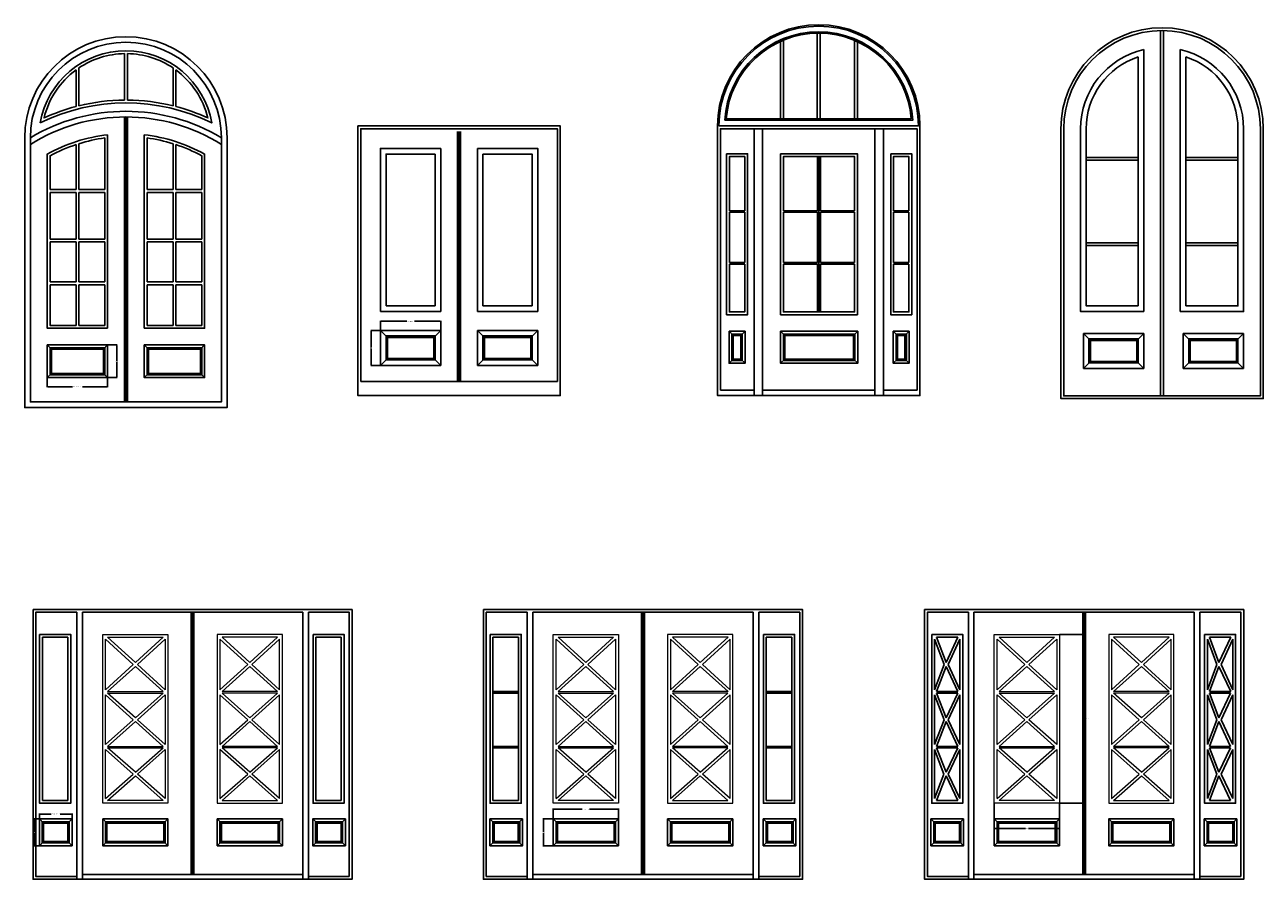
# Model space of a CAD drawing. Units: inches. Extents: x 1451 to 1892, y 1255 to 1559.
import ezdxf

# ---------------------------------------------------------------- set-up
doc = ezdxf.new("R2010")
doc.units = ezdxf.units.IN
doc.header["$MEASUREMENT"] = 0
for name, color, linetype, lineweight in [('A-ANNO-DIMS', 2, 'Continuous', 18), ('A-DOOR', 4, 'Continuous', 25), ('A-GLAZ', 3, 'Continuous', 18)]:
    doc.layers.add(name, color=color, linetype=linetype, lineweight=lineweight)
doc.styles.get("Standard").update_dxf_attribs({"font": 'arial.ttf'})
doc.dimstyles.get("Standard").update_dxf_attribs({"dimtxt": 0.18, "dimasz": 0.18, "dimexe": 0.18, "dimexo": 0.0625, "dimgap": 0.09, "dimtad": 0, "dimtih": 1, "dimtoh": 1, "dimdec": 4, "dimzin": 0, "dimdsep": 46, "dimtxsty": 'Standard', "dimcen": 0.09, "dimadec": 0, "dimazin": 0, "dimtfac": 1, "dimtdec": 4, "dimtofl": 0, "dimtmove": 0, "dimatfit": 3, "dimfxl": 1, "dimtolj": 1, "dimtzin": 0, "dimarcsym": 0})

# ---------------------------------------------------------------- blocks, each defined once
blk = doc.blocks.new('GLAZ-X-MUNTIN')
for p, q in [((1489.65, 1331.77), (1479.78, 1340.77)), ((1490.39, 1332.44), (1480.52, 1341.44)), ((1490.39, 1332.44), (1500.26, 1341.44)), ((1491.13, 1331.77), (1501, 1340.77)), ((1479.78, 1322.77), (1489.65, 1331.77)), ((1480.52, 1322.09), (1490.39, 1331.09)), ((1500.26, 1322.09), (1490.39, 1331.09)), ((1501, 1322.77), (1491.13, 1331.77)), ((1480.52, 1322.09), (1500.26, 1322.09)), ((1489.64, 1312.11), (1479.78, 1320.92)), ((1480.53, 1321.59), (1500.25, 1321.59)), ((1490.39, 1312.78), (1480.53, 1321.59)), ((1490.39, 1312.78), (1500.25, 1321.59)), ((1491.14, 1312.11), (1501, 1320.92)), ((1479.78, 1303.29), (1489.64, 1312.11)), ((1480.53, 1302.62), (1490.39, 1311.44)), ((1500.25, 1302.62), (1490.39, 1311.44)), ((1501, 1303.29), (1491.14, 1312.11)), ((1489.64, 1292.74), (1479.78, 1301.46)), ((1480.53, 1302.62), (1500.25, 1302.62)), ((1480.54, 1302.12), (1500.24, 1302.12)), ((1490.39, 1293.41), (1480.54, 1302.12)), ((1490.39, 1293.41), (1500.24, 1302.12)), ((1491.14, 1292.74), (1501, 1301.46)), ((1479.78, 1284.02), (1489.64, 1292.74)), ((1480.54, 1283.35), (1490.39, 1292.07)), ((1500.24, 1283.35), (1490.39, 1292.07)), ((1501, 1284.02), (1491.14, 1292.74))]:
    blk.add_line(p, q)
blk.add_lwpolyline([(1478.78, 1342.44), (1502, 1342.44), (1502, 1282.35), (1478.78, 1282.35)], close=True)
for points in [[(1479.78, 1322.77), (1479.78, 1340.77)], [(1480.52, 1341.44), (1500.26, 1341.44)], [(1501, 1340.77), (1501, 1322.77)], [(1479.78, 1303.29), (1479.78, 1320.92)], [(1501, 1320.92), (1501, 1303.29)], [(1479.78, 1284.02), (1479.78, 1301.46)], [(1501, 1301.46), (1501, 1284.02)], [(1500.24, 1283.35), (1480.54, 1283.35)]]:
    blk.add_lwpolyline(points)
blk = doc.blocks.new('PANEL-RAISED-LEAF')
for p, q in [((1478.78, 1276.79), (1480.28, 1275.29)), ((1502, 1276.79), (1500.5, 1275.29)), ((1478.78, 1267.24), (1480.28, 1268.74)), ((1500.5, 1268.74), (1502, 1267.24))]:
    blk.add_line(p, q)
for points in [[(1478.78, 1276.79), (1502, 1276.79), (1502, 1267.24), (1478.78, 1267.24)], [(1479.78, 1275.79), (1501, 1275.79), (1501, 1268.24), (1479.78, 1268.24)], [(1480.28, 1275.29), (1500.5, 1275.29), (1500.5, 1268.74), (1480.28, 1268.74)]]:
    blk.add_lwpolyline(points, close=True)
blk = doc.blocks.new('PANEL-RAISED-SIDELT')
for p, q in [((1456.26, 1276.79), (1457.76, 1275.29)), ((1467.87, 1276.79), (1466.37, 1275.29)), ((1456.26, 1267.24), (1457.76, 1268.74)), ((1467.87, 1267.24), (1466.37, 1268.74))]:
    blk.add_line(p, q)
for points in [[(1467.87, 1276.79), (1456.26, 1276.79), (1456.26, 1267.24), (1467.87, 1267.24)], [(1466.87, 1275.79), (1457.26, 1275.79), (1457.26, 1268.24), (1466.87, 1268.24)], [(1466.37, 1275.29), (1457.76, 1275.29), (1457.76, 1268.74), (1466.37, 1268.74)]]:
    blk.add_lwpolyline(points, close=True)
blk = doc.blocks.new('PANEL-RAISED-ARCH')
for p, q in [((1459.04, 1445.5), (1460.54, 1444)), ((1480.54, 1445.5), (1479.04, 1444)), ((1459.04, 1433.86), (1460.54, 1435.36)), ((1480.54, 1433.86), (1479.04, 1435.36))]:
    blk.add_line(p, q)
for points in [[(1459.04, 1445.5), (1480.54, 1445.5), (1480.54, 1433.86), (1459.04, 1433.86)], [(1460.04, 1444.5), (1479.54, 1444.5), (1479.54, 1434.86), (1460.04, 1434.86)], [(1460.54, 1444), (1479.04, 1444), (1479.04, 1435.36), (1460.54, 1435.36)]]:
    blk.add_lwpolyline(points, close=True)
blk = doc.blocks.new('PANEL-RAISED-DEEP')
for p, q in [((0, 12.55), (21.5, 12.55)), ((2.5, 10.05), (0, 12.55)), ((21.5, 12.55), (19, 10.05)), ((21.5, 0), (21.5, 12.55)), ((0, 0), (2.5, 2.5)), ((0, 0), (21.5, 0)), ((21.5, 0), (19, 2.5))]:
    blk.add_line(p, q)
blk.add_lwpolyline([(0, 0), (0, 12.55)])
blk.add_lwpolyline([(19, 10.05), (19, 2.5), (2.5, 2.5), (2.5, 10.05)], close=True)
blk = doc.blocks.new('*D6')
at = {"layer": 'A-ANNO-DIMS', "color": 0, "lineweight": -2, "transparency": 16777216}
for p, q in [((1819.28, 1342.44), (1828.41, 1342.44)), ((1828.23, 1342.26), (1828.23, 1312.58)), ((1828.23, 1282.53), (1828.23, 1312.22)), ((1819.28, 1282.35), (1828.41, 1282.35))]:
    blk.add_line(p, q, dxfattribs=at)
at = {"layer": 'A-ANNO-DIMS', "color": 0, "transparency": 16777216}
for points in [[(1828.2, 1342.26), (1828.26, 1342.26), (1828.23, 1342.44)], [(1828.2, 1282.53), (1828.26, 1282.53), (1828.23, 1282.35)]]:
    blk.add_solid(points, dxfattribs=at)
at = {"layer": 'Defpoints', "color": 0, "transparency": 16777216}
for p in [(1819.22, 1342.44), (1828.23, 1342.44), (1819.22, 1282.35)]:
    blk.add_point(p, dxfattribs=at)
at = {"layer": 'A-ANNO-DIMS', "color": 0, "transparency": 16777216, "insert": (1828.23, 1312.4), "char_height": 0.18, "attachment_point": 5}
blk.add_mtext('\\A1;X-MUNTIN LITE 60 TYP.', dxfattribs=at)
blk = doc.blocks.new('*D7')
at = {"layer": 'A-ANNO-DIMS', "color": 0, "lineweight": -2, "transparency": 16777216}
for p, q in [((1796.01, 1282.29), (1796.01, 1273.16)), ((1819.22, 1282.29), (1819.22, 1273.16)), ((1796.19, 1273.34), (1807.08, 1273.34)), ((1819.04, 1273.34), (1808.14, 1273.34))]:
    blk.add_line(p, q, dxfattribs=at)
at = {"layer": 'A-ANNO-DIMS', "color": 0, "transparency": 16777216}
for points in [[(1796.19, 1273.37), (1796.19, 1273.31), (1796.01, 1273.34)], [(1819.04, 1273.37), (1819.04, 1273.31), (1819.22, 1273.34)]]:
    blk.add_solid(points, dxfattribs=at)
at = {"layer": 'Defpoints', "color": 0, "transparency": 16777216}
for p in [(1796.01, 1282.35), (1819.22, 1282.35), (1819.22, 1273.34)]:
    blk.add_point(p, dxfattribs=at)
at = {"layer": 'A-ANNO-DIMS', "color": 0, "transparency": 16777216, "insert": (1807.61, 1273.34), "char_height": 0.18, "attachment_point": 5}
blk.add_mtext('\\A1;23 TYP.', dxfattribs=at)
blk = doc.blocks.new('*D8')
at = {"layer": 'A-ANNO-DIMS', "color": 0, "lineweight": -2, "transparency": 16777216}
for p, q in [((1639.07, 1276.85), (1639.07, 1280.45)), ((1639.25, 1280.27), (1649.36, 1280.27)), ((1662.11, 1280.27), (1652, 1280.27)), ((1662.29, 1276.85), (1662.29, 1280.45))]:
    blk.add_line(p, q, dxfattribs=at)
at = {"layer": 'A-ANNO-DIMS', "color": 0, "transparency": 16777216}
for points in [[(1639.25, 1280.3), (1639.25, 1280.24), (1639.07, 1280.27)], [(1662.11, 1280.3), (1662.11, 1280.24), (1662.29, 1280.27)]]:
    blk.add_solid(points, dxfattribs=at)
at = {"layer": 'Defpoints', "color": 0, "transparency": 16777216}
for p in [(1662.29, 1280.27), (1639.07, 1276.79), (1662.29, 1276.79)]:
    blk.add_point(p, dxfattribs=at)
at = {"layer": 'A-ANNO-DIMS', "color": 0, "transparency": 16777216, "insert": (1650.68, 1280.27), "char_height": 0.18, "attachment_point": 5}
blk.add_mtext('\\A1;LEAF PANEL 23 TYP.', dxfattribs=at)
blk = doc.blocks.new('*D9')
at = {"layer": 'A-ANNO-DIMS', "color": 0, "lineweight": -2, "transparency": 16777216}
for p, q in [((1639.01, 1276.79), (1635.41, 1276.79)), ((1635.59, 1276.61), (1635.59, 1272.2)), ((1635.59, 1267.42), (1635.59, 1271.83)), ((1639.01, 1267.24), (1635.41, 1267.24))]:
    blk.add_line(p, q, dxfattribs=at)
at = {"layer": 'A-ANNO-DIMS', "color": 0, "transparency": 16777216}
for points in [[(1635.56, 1276.61), (1635.62, 1276.61), (1635.59, 1276.79)], [(1635.56, 1267.42), (1635.62, 1267.42), (1635.59, 1267.24)]]:
    blk.add_solid(points, dxfattribs=at)
at = {"layer": 'Defpoints', "color": 0, "transparency": 16777216}
for p in [(1635.59, 1276.79), (1639.07, 1276.79), (1639.07, 1267.24)]:
    blk.add_point(p, dxfattribs=at)
at = {"layer": 'A-ANNO-DIMS', "color": 0, "transparency": 16777216, "insert": (1635.59, 1272.02), "char_height": 0.18, "attachment_point": 5}
blk.add_mtext('\\A1;10 TYP.', dxfattribs=at)
blk = doc.blocks.new('*D10')
at = {"layer": 'A-ANNO-DIMS', "color": 0, "lineweight": -2, "transparency": 16777216}
for p, q in [((1456.26, 1276.85), (1456.26, 1278.71)), ((1456.44, 1278.53), (1460.49, 1278.53)), ((1467.69, 1278.53), (1463.63, 1278.53)), ((1467.87, 1276.85), (1467.87, 1278.71))]:
    blk.add_line(p, q, dxfattribs=at)
at = {"layer": 'A-ANNO-DIMS', "color": 0, "transparency": 16777216}
for points in [[(1456.44, 1278.56), (1456.44, 1278.5), (1456.26, 1278.53)], [(1467.69, 1278.56), (1467.69, 1278.5), (1467.87, 1278.53)]]:
    blk.add_solid(points, dxfattribs=at)
at = {"layer": 'Defpoints', "color": 0, "transparency": 16777216}
for p in [(1467.87, 1278.53), (1456.26, 1276.79), (1467.87, 1276.79)]:
    blk.add_point(p, dxfattribs=at)
at = {"layer": 'A-ANNO-DIMS', "color": 0, "transparency": 16777216, "insert": (1462.06, 1278.53), "char_height": 0.18, "attachment_point": 5}
blk.add_mtext('\\A1;SIDELITE PANEL 12 TYP.', dxfattribs=at)
blk = doc.blocks.new('*D11')
at = {"layer": 'A-ANNO-DIMS', "color": 0, "lineweight": -2, "transparency": 16777216}
for p, q in [((1456.2, 1276.79), (1454.34, 1276.79)), ((1454.52, 1276.61), (1454.52, 1272.2)), ((1454.52, 1267.42), (1454.52, 1271.83)), ((1456.2, 1267.24), (1454.34, 1267.24))]:
    blk.add_line(p, q, dxfattribs=at)
at = {"layer": 'A-ANNO-DIMS', "color": 0, "transparency": 16777216}
for points in [[(1454.49, 1276.61), (1454.55, 1276.61), (1454.52, 1276.79)], [(1454.49, 1267.42), (1454.55, 1267.42), (1454.52, 1267.24)]]:
    blk.add_solid(points, dxfattribs=at)
at = {"layer": 'Defpoints', "color": 0, "transparency": 16777216}
for p in [(1454.52, 1276.79), (1456.26, 1276.79), (1456.26, 1267.24)]:
    blk.add_point(p, dxfattribs=at)
at = {"layer": 'A-ANNO-DIMS', "color": 0, "transparency": 16777216, "insert": (1454.52, 1272.02), "char_height": 0.18, "attachment_point": 5}
blk.add_mtext('\\A1;10 TYP.', dxfattribs=at)
blk = doc.blocks.new('*D12')
at = {"layer": 'A-ANNO-DIMS', "color": 0, "lineweight": -2, "transparency": 16777216}
for p, q in [((1577.58, 1450.74), (1577.58, 1454.09)), ((1577.76, 1453.91), (1586.98, 1453.91)), ((1598.9, 1453.91), (1589.68, 1453.91)), ((1599.08, 1450.74), (1599.08, 1454.09))]:
    blk.add_line(p, q, dxfattribs=at)
at = {"layer": 'A-ANNO-DIMS', "color": 0, "transparency": 16777216}
for points in [[(1577.76, 1453.94), (1577.76, 1453.88), (1577.58, 1453.91)], [(1598.9, 1453.94), (1598.9, 1453.88), (1599.08, 1453.91)]]:
    blk.add_solid(points, dxfattribs=at)
at = {"layer": 'Defpoints', "color": 0, "transparency": 16777216}
for p in [(1577.58, 1450.68), (1599.08, 1453.91), (1599.08, 1450.68)]:
    blk.add_point(p, dxfattribs=at)
at = {"layer": 'A-ANNO-DIMS', "color": 0, "transparency": 16777216, "insert": (1588.33, 1453.91), "char_height": 0.18, "attachment_point": 5}
blk.add_mtext('\\A1;DEEP PANEL 22 TYP.', dxfattribs=at)
blk = doc.blocks.new('*D13')
at = {"layer": 'A-ANNO-DIMS', "color": 0, "lineweight": -2, "transparency": 16777216}
for p, q in [((1577.52, 1450.68), (1574.18, 1450.68)), ((1574.36, 1450.5), (1574.36, 1444.59)), ((1574.36, 1438.31), (1574.36, 1444.22)), ((1577.52, 1438.13), (1574.18, 1438.13))]:
    blk.add_line(p, q, dxfattribs=at)
at = {"layer": 'A-ANNO-DIMS', "color": 0, "transparency": 16777216}
for points in [[(1574.33, 1450.5), (1574.39, 1450.5), (1574.36, 1450.68)], [(1574.33, 1438.31), (1574.39, 1438.31), (1574.36, 1438.13)]]:
    blk.add_solid(points, dxfattribs=at)
at = {"layer": 'Defpoints', "color": 0, "transparency": 16777216}
for p in [(1574.36, 1450.68), (1577.58, 1450.68), (1577.58, 1438.13)]:
    blk.add_point(p, dxfattribs=at)
at = {"layer": 'A-ANNO-DIMS', "color": 0, "transparency": 16777216, "insert": (1574.36, 1444.4), "char_height": 0.18, "attachment_point": 5}
blk.add_mtext('\\A1;13 TYP.', dxfattribs=at)
blk = doc.blocks.new('*D14')
at = {"layer": 'A-ANNO-DIMS', "color": 0, "lineweight": -2, "transparency": 16777216}
for p, q in [((1459.04, 1433.8), (1459.04, 1430.45)), ((1480.54, 1433.8), (1480.54, 1430.45)), ((1459.22, 1430.63), (1468, 1430.63)), ((1480.36, 1430.63), (1471.59, 1430.63))]:
    blk.add_line(p, q, dxfattribs=at)
at = {"layer": 'A-ANNO-DIMS', "color": 0, "transparency": 16777216}
for points in [[(1459.22, 1430.66), (1459.22, 1430.6), (1459.04, 1430.63)], [(1480.36, 1430.66), (1480.36, 1430.6), (1480.54, 1430.63)]]:
    blk.add_solid(points, dxfattribs=at)
at = {"layer": 'Defpoints', "color": 0, "transparency": 16777216}
for p in [(1459.04, 1433.86), (1480.54, 1433.86), (1480.54, 1430.63)]:
    blk.add_point(p, dxfattribs=at)
at = {"layer": 'A-ANNO-DIMS', "color": 0, "transparency": 16777216, "insert": (1469.79, 1430.63), "char_height": 0.18, "attachment_point": 5}
blk.add_mtext('\\A1;ARCH-DOOR PANEL 22 TYP.', dxfattribs=at)
blk = doc.blocks.new('*D15')
at = {"layer": 'A-ANNO-DIMS', "color": 0, "lineweight": -2, "transparency": 16777216}
for p, q in [((1480.61, 1445.5), (1483.95, 1445.5)), ((1483.77, 1445.32), (1483.77, 1439.86)), ((1483.77, 1434.04), (1483.77, 1439.5)), ((1480.61, 1433.86), (1483.95, 1433.86))]:
    blk.add_line(p, q, dxfattribs=at)
at = {"layer": 'A-ANNO-DIMS', "color": 0, "transparency": 16777216}
for points in [[(1483.74, 1445.32), (1483.8, 1445.32), (1483.77, 1445.5)], [(1483.74, 1434.04), (1483.8, 1434.04), (1483.77, 1433.86)]]:
    blk.add_solid(points, dxfattribs=at)
at = {"layer": 'Defpoints', "color": 0, "transparency": 16777216}
for p in [(1480.54, 1445.5), (1483.77, 1445.5), (1480.54, 1433.86)]:
    blk.add_point(p, dxfattribs=at)
at = {"layer": 'A-ANNO-DIMS', "color": 0, "transparency": 16777216, "insert": (1483.77, 1439.68), "char_height": 0.18, "attachment_point": 5}
blk.add_mtext('\\A1;12 TYP.', dxfattribs=at)

msp = doc.modelspace()

# ---------------------------------------------------------------- linework, layer by layer
at = {"layer": 'A-DOOR'}
for p, q in [((1733.02, 1525.94), (1733.02, 1556.44)), ((1734.02, 1525.94), (1734.02, 1556.44)), ((1855.22, 1427.37), (1855.22, 1557.37)), ((1856.22, 1427.37), (1856.22, 1557.37)), ((1720, 1525.94), (1720, 1553.53)), ((1721, 1525.94), (1721, 1553.96)), ((1746.3, 1525.94), (1746.3, 1553.88)), ((1747.3, 1525.94), (1747.3, 1553.44)), ((1486.54, 1532.64), (1486.54, 1549.18)), ((1487.54, 1532.64), (1487.54, 1549.18)), ((1847.22, 1459.35), (1847.22, 1548)), ((1849.22, 1457.35), (1849.22, 1550.64)), ((1862.22, 1457.35), (1862.22, 1550.64)), ((1864.22, 1459.35), (1864.22, 1548)), ((1469.29, 1530.35), (1469.29, 1543.37)), ((1470.29, 1530.6), (1470.29, 1544.07)), ((1503.79, 1530.6), (1503.79, 1544.07)), ((1504.79, 1530.35), (1504.79, 1543.37)), ((1486.54, 1425.19), (1486.54, 1526.64)), ((1487.04, 1425.19), (1487.04, 1526.64)), ((1487.54, 1425.19), (1487.54, 1526.64)), ((1605.08, 1432.47), (1605.08, 1521.44)), ((1605.58, 1432.47), (1605.58, 1521.44)), ((1605.58, 1432.47), (1605.58, 1521.44)), ((1606.08, 1432.47), (1606.08, 1521.44)), ((1710.55, 1522.44), (1710.55, 1427.44)), ((1713.55, 1522.44), (1713.55, 1427.44)), ((1753.55, 1522.44), (1753.55, 1427.44)), ((1756.55, 1522.44), (1756.55, 1427.44)), ((1453.04, 1516.84), (1453.04, 1519.19)), ((1469.29, 1500.78), (1469.29, 1516.8)), ((1470.29, 1500.78), (1470.29, 1517.12)), ((1479.54, 1500.78), (1479.54, 1519.15)), ((1480.54, 1451.45), (1480.54, 1520.28)), ((1493.54, 1451.45), (1493.54, 1520.28)), ((1494.54, 1500.78), (1494.54, 1519.15)), ((1503.79, 1500.78), (1503.79, 1517.12)), ((1504.79, 1500.78), (1504.79, 1516.8)), ((1521.04, 1516.84), (1521.04, 1519.19)), ((1597.08, 1459.35), (1597.08, 1513.44)), ((1599.08, 1457.35), (1599.08, 1515.44)), ((1612.08, 1457.35), (1612.08, 1515.44)), ((1614.08, 1459.35), (1614.08, 1513.44)), ((1700.76, 1493.22), (1700.76, 1512.55)), ((1701.76, 1493.22), (1701.76, 1512.55)), ((1733.15, 1493.22), (1733.15, 1512.55)), ((1733.65, 1457.21), (1733.65, 1512.55)), ((1734.15, 1493.22), (1734.15, 1512.55)), ((1759.16, 1493.22), (1759.16, 1512.55)), ((1760.16, 1493.22), (1760.16, 1512.55)), ((1828.72, 1512.2), (1847.22, 1512.2)), ((1864.22, 1512.2), (1882.72, 1512.2)), ((1828.72, 1511.2), (1847.22, 1511.2)), ((1864.22, 1511.2), (1882.72, 1511.2)), ((1460.04, 1500.78), (1469.29, 1500.78)), ((1460.04, 1499.78), (1469.29, 1499.78)), ((1469.29, 1483.13), (1469.29, 1499.78)), ((1470.29, 1500.78), (1479.54, 1500.78)), ((1470.29, 1499.78), (1479.54, 1499.78)), ((1470.29, 1483.13), (1470.29, 1499.78)), ((1479.54, 1483.13), (1479.54, 1499.78)), ((1494.54, 1500.78), (1503.79, 1500.78)), ((1494.54, 1499.78), (1503.79, 1499.78)), ((1494.54, 1483.13), (1494.54, 1499.78)), ((1503.79, 1483.13), (1503.79, 1499.78)), ((1504.79, 1500.78), (1514.04, 1500.78)), ((1504.79, 1483.13), (1504.79, 1499.78)), ((1504.79, 1499.78), (1514.04, 1499.78)), ((1700.76, 1474.77), (1700.76, 1492.72)), ((1701.76, 1493.22), (1707.24, 1493.22)), ((1701.76, 1474.77), (1701.76, 1492.72)), ((1701.76, 1492.72), (1707.24, 1492.72)), ((1721, 1493.22), (1733.15, 1493.22)), ((1721, 1492.72), (1733.15, 1492.72)), ((1733.15, 1474.77), (1733.15, 1492.72)), ((1734.15, 1493.22), (1746.3, 1493.22)), ((1734.15, 1474.77), (1734.15, 1492.72)), ((1734.15, 1492.72), (1746.3, 1492.72)), ((1759.16, 1474.77), (1759.16, 1492.72)), ((1760.16, 1493.22), (1765.64, 1493.22)), ((1760.16, 1474.77), (1760.16, 1492.72)), ((1760.16, 1492.72), (1765.64, 1492.72)), ((1460.04, 1483.13), (1469.29, 1483.13)), ((1460.04, 1482.13), (1469.29, 1482.13)), ((1469.29, 1467.9), (1469.29, 1482.13)), ((1470.29, 1483.13), (1479.54, 1483.13)), ((1470.29, 1482.13), (1479.54, 1482.13)), ((1470.29, 1467.9), (1470.29, 1482.13)), ((1479.54, 1467.9), (1479.54, 1482.13)), ((1494.54, 1483.13), (1503.79, 1483.13)), ((1494.54, 1482.13), (1503.79, 1482.13)), ((1494.54, 1467.9), (1494.54, 1482.13)), ((1503.79, 1467.9), (1503.79, 1482.13)), ((1504.79, 1483.13), (1514.04, 1483.13)), ((1504.79, 1467.9), (1504.79, 1482.13)), ((1504.79, 1482.13), (1514.04, 1482.13)), ((1828.72, 1481.84), (1847.22, 1481.84)), ((1828.72, 1480.84), (1847.22, 1480.84)), ((1864.22, 1481.84), (1882.72, 1481.84)), ((1864.22, 1480.84), (1882.72, 1480.84)), ((1700.76, 1457.21), (1700.76, 1474.27)), ((1701.76, 1474.77), (1707.24, 1474.77)), ((1701.76, 1457.21), (1701.76, 1474.27)), ((1701.76, 1474.27), (1707.24, 1474.27)), ((1721, 1474.77), (1733.15, 1474.77)), ((1721, 1474.27), (1733.15, 1474.27)), ((1733.15, 1457.21), (1733.15, 1474.27)), ((1734.15, 1474.77), (1746.3, 1474.77)), ((1734.15, 1457.21), (1734.15, 1474.27)), ((1734.15, 1474.27), (1746.3, 1474.27)), ((1759.16, 1457.21), (1759.16, 1474.27)), ((1760.16, 1474.77), (1765.64, 1474.77)), ((1760.16, 1457.21), (1760.16, 1474.27)), ((1760.16, 1474.27), (1765.64, 1474.27)), ((1460.04, 1467.9), (1469.29, 1467.9)), ((1470.29, 1467.9), (1479.54, 1467.9)), ((1494.54, 1467.9), (1503.79, 1467.9)), ((1504.79, 1467.9), (1514.04, 1467.9)), ((1460.04, 1466.9), (1469.29, 1466.9)), ((1469.29, 1452.45), (1469.29, 1466.9)), ((1470.29, 1452.45), (1470.29, 1466.9)), ((1470.29, 1466.9), (1479.54, 1466.9)), ((1479.54, 1452.45), (1479.54, 1466.9)), ((1494.54, 1452.45), (1494.54, 1466.9)), ((1494.54, 1466.9), (1503.79, 1466.9)), ((1503.79, 1452.45), (1503.79, 1466.9)), ((1504.79, 1452.45), (1504.79, 1466.9)), ((1504.79, 1466.9), (1514.04, 1466.9)), ((1579.58, 1459.35), (1597.08, 1459.35)), ((1614.08, 1459.35), (1631.58, 1459.35)), ((1577.58, 1457.35), (1599.08, 1457.35)), ((1612.08, 1457.35), (1633.58, 1457.35)), ((1703.16, 1448.84), (1701.66, 1450.34)), ((1705.83, 1448.84), (1707.33, 1450.34)), ((1721.5, 1448.84), (1720, 1450.34)), ((1745.92, 1448.84), (1747.42, 1450.34)), ((1761.56, 1448.84), (1760.06, 1450.34)), ((1764.23, 1448.84), (1765.73, 1450.34)), ((1701.66, 1438.95), (1703.16, 1440.45)), ((1705.83, 1440.45), (1707.33, 1438.95)), ((1720, 1438.95), (1721.5, 1440.45)), ((1745.92, 1440.45), (1747.42, 1438.95)), ((1760.06, 1438.95), (1761.56, 1440.45)), ((1764.23, 1440.45), (1765.73, 1438.95)), ((1570.58, 1432.47), (1640.58, 1432.47)), ((1698.55, 1429.43), (1710.55, 1429.43)), ((1713.55, 1429.43), (1753.55, 1429.43)), ((1756.55, 1429.43), (1768.55, 1429.43)), ((1469.56, 1255.32), (1469.56, 1350.32)), ((1471.56, 1255.32), (1471.56, 1350.32)), ((1510.26, 1257.04), (1510.26, 1350.32)), ((1510.76, 1257.04), (1510.76, 1350.32)), ((1510.76, 1257.04), (1510.76, 1350.32)), ((1510.76, 1257.04), (1510.76, 1350.32)), ((1511.26, 1257.04), (1511.26, 1350.32)), ((1549.95, 1255.32), (1549.95, 1350.32)), ((1551.95, 1255.32), (1551.95, 1350.32)), ((1629.85, 1255.32), (1629.85, 1350.32)), ((1631.85, 1255.32), (1631.85, 1350.32)), ((1670.55, 1257.04), (1670.55, 1350.32)), ((1671.05, 1257.04), (1671.05, 1350.32)), ((1671.05, 1257.04), (1671.05, 1350.32)), ((1671.05, 1257.04), (1671.05, 1350.32)), ((1671.55, 1257.04), (1671.55, 1350.32)), ((1710.24, 1255.32), (1710.24, 1350.32)), ((1712.24, 1255.32), (1712.24, 1350.32)), ((1786.79, 1255.32), (1786.79, 1350.32)), ((1788.79, 1255.32), (1788.79, 1350.32)), ((1827.48, 1257.04), (1827.48, 1350.32)), ((1827.98, 1257.04), (1827.98, 1350.32)), ((1827.98, 1257.04), (1827.98, 1350.32)), ((1827.98, 1257.04), (1827.98, 1350.32)), ((1828.48, 1257.04), (1828.48, 1350.32)), ((1867.17, 1255.32), (1867.17, 1350.32)), ((1869.17, 1255.32), (1869.17, 1350.32)), ((1457.34, 1341.44), (1458.08, 1341.44)), ((1554.61, 1340.77), (1554.61, 1341.44)), ((1554.61, 1341.44), (1555.36, 1341.44)), ((1562.92, 1341.44), (1563.66, 1341.44)), ((1563.66, 1341.44), (1563.66, 1340.77)), ((1617.63, 1341.44), (1618.38, 1341.44)), ((1714.9, 1340.77), (1714.9, 1341.44)), ((1714.9, 1341.44), (1715.65, 1341.44)), ((1723.21, 1341.44), (1723.95, 1341.44)), ((1723.95, 1341.44), (1723.95, 1340.77)), ((1778.13, 1331.77), (1774.75, 1340.77)), ((1778.88, 1332.44), (1775.49, 1341.44)), ((1778.88, 1332.44), (1783.05, 1341.44)), ((1779.62, 1331.77), (1783.8, 1340.77)), ((1875.22, 1331.77), (1871.84, 1340.77)), ((1875.96, 1332.44), (1872.58, 1341.44)), ((1875.96, 1332.44), (1880.14, 1341.44)), ((1876.71, 1331.77), (1880.88, 1340.77)), ((1774.75, 1322.77), (1778.13, 1331.77)), ((1775.49, 1322.09), (1778.88, 1331.09)), ((1783.05, 1322.09), (1778.88, 1331.09)), ((1783.8, 1322.77), (1779.62, 1331.77)), ((1871.84, 1322.77), (1875.22, 1331.77)), ((1872.58, 1322.09), (1875.96, 1331.09)), ((1880.14, 1322.09), (1875.96, 1331.09)), ((1880.88, 1322.77), (1876.71, 1331.77)), ((1617.63, 1322.09), (1626.68, 1322.09)), ((1714.9, 1322.09), (1723.95, 1322.09)), ((1775.49, 1322.09), (1783.05, 1322.09)), ((1872.58, 1322.09), (1880.14, 1322.09)), ((1617.63, 1321.59), (1626.68, 1321.59)), ((1714.9, 1321.59), (1723.95, 1321.59)), ((1778.13, 1312.11), (1774.75, 1320.92)), ((1775.5, 1321.59), (1783.05, 1321.59)), ((1778.88, 1312.78), (1775.5, 1321.59)), ((1778.88, 1312.78), (1783.05, 1321.59)), ((1779.63, 1312.11), (1783.8, 1320.92)), ((1875.21, 1312.11), (1871.84, 1320.92)), ((1872.59, 1321.59), (1880.13, 1321.59)), ((1875.96, 1312.78), (1872.59, 1321.59)), ((1875.96, 1312.78), (1880.13, 1321.59)), ((1876.71, 1312.11), (1880.88, 1320.92)), ((1774.75, 1303.29), (1778.13, 1312.11)), ((1775.5, 1302.62), (1778.88, 1311.44)), ((1783.05, 1302.62), (1778.88, 1311.44)), ((1783.8, 1303.29), (1779.63, 1312.11)), ((1871.84, 1303.29), (1875.21, 1312.11)), ((1872.59, 1302.62), (1875.96, 1311.44)), ((1880.13, 1302.62), (1875.96, 1311.44)), ((1880.88, 1303.29), (1876.71, 1312.11)), ((1617.63, 1302.62), (1626.68, 1302.62)), ((1617.63, 1302.12), (1626.68, 1302.12)), ((1714.9, 1302.62), (1723.95, 1302.62)), ((1714.9, 1302.12), (1723.95, 1302.12)), ((1778.12, 1292.74), (1774.75, 1301.46)), ((1775.5, 1302.62), (1783.05, 1302.62)), ((1775.5, 1302.12), (1783.04, 1302.12)), ((1778.88, 1293.41), (1775.5, 1302.12)), ((1778.88, 1293.41), (1783.04, 1302.12)), ((1779.63, 1292.74), (1783.8, 1301.46)), ((1875.21, 1292.74), (1871.84, 1301.46)), ((1872.59, 1302.62), (1880.13, 1302.62)), ((1872.59, 1302.12), (1880.13, 1302.12)), ((1875.96, 1293.41), (1872.59, 1302.12)), ((1875.96, 1293.41), (1880.13, 1302.12)), ((1876.72, 1292.74), (1880.88, 1301.46)), ((1774.75, 1284.02), (1778.12, 1292.74)), ((1775.5, 1283.35), (1778.88, 1292.07)), ((1783.04, 1283.35), (1778.88, 1292.07)), ((1783.8, 1284.02), (1779.63, 1292.74)), ((1871.84, 1284.02), (1875.21, 1292.74)), ((1872.59, 1283.35), (1875.96, 1292.07)), ((1880.13, 1283.35), (1875.96, 1292.07)), ((1880.88, 1284.02), (1876.72, 1292.74)), ((1457.34, 1284.02), (1457.34, 1283.35)), ((1457.34, 1283.35), (1458.1, 1283.35)), ((1465.64, 1283.35), (1466.39, 1283.35)), ((1466.39, 1283.35), (1466.39, 1284.02)), ((1554.61, 1284.02), (1554.61, 1283.35)), ((1554.61, 1283.35), (1555.37, 1283.35)), ((1562.91, 1283.35), (1563.66, 1283.35)), ((1563.66, 1283.35), (1563.66, 1284.02)), ((1617.63, 1284.02), (1617.63, 1283.35)), ((1617.63, 1283.35), (1618.39, 1283.35)), ((1625.93, 1283.35), (1626.68, 1283.35)), ((1626.68, 1283.35), (1626.68, 1284.02)), ((1714.9, 1284.02), (1714.9, 1283.35)), ((1714.9, 1283.35), (1715.66, 1283.35)), ((1723.2, 1283.35), (1723.95, 1283.35)), ((1723.95, 1283.35), (1723.95, 1284.02)), ((1471.56, 1257.04), (1549.95, 1257.04)), ((1566.53, 1256.32), (1551.95, 1256.32)), ((1631.85, 1257.04), (1710.24, 1257.04)), ((1726.83, 1256.32), (1712.24, 1256.32)), ((1788.79, 1257.04), (1867.17, 1257.04)), ((1883.76, 1256.32), (1869.17, 1256.32))]:
    msp.add_line(p, q, dxfattribs=at)
for points in [[(1891.72, 1522.37), (1891.72, 1426.37), (1819.72, 1426.37), (1819.72, 1522.37, -1)], [(1890.72, 1522.37), (1890.72, 1427.37), (1820.72, 1427.37), (1820.72, 1522.37, -1)], [(1523.04, 1519.19), (1523.04, 1423.19), (1451.04, 1423.19), (1451.04, 1519.19, -1)], [(1453.04, 1519.19, -1), (1521.04, 1519.19, 0.27814)], [(1456.5, 1524.5, -0.841089), (1517.59, 1524.5, 0.233941)]]:
    msp.add_lwpolyline(points, format="xyb", close=True, dxfattribs=at)
for points in [[(1470.29, 1544.07, -0.144929), (1486.54, 1549.18, -0.144929)], [(1487.54, 1549.18, -0.144929), (1503.79, 1544.07)], [(1849.22, 1457.35), (1826.72, 1457.35), (1826.72, 1522.37, -0.34945), (1849.22, 1550.64)], [(1847.22, 1459.35), (1828.72, 1459.35), (1828.72, 1522.37, -0.323234), (1847.22, 1548)], [(1862.22, 1550.64, -0.34945), (1884.72, 1522.37), (1884.72, 1457.35), (1862.22, 1457.35)], [(1864.22, 1548, -0.323234), (1882.72, 1522.37), (1882.72, 1459.35), (1864.22, 1459.35)], [(1469.29, 1530.35, 0.043427), (1457.89, 1526.27, -0.176638), (1469.29, 1543.37, -0.176638)], [(1504.79, 1543.37, -0.176638), (1516.2, 1526.27, 0.043427), (1504.79, 1530.35, 0.043427)], [(1486.54, 1532.64, 0.058819), (1470.29, 1530.6)], [(1503.79, 1530.6, 0.058819), (1487.54, 1532.64, 0.058819)], [(1487.04, 1526.64, -0.14132), (1521.04, 1516.84), (1521.04, 1425.19), (1453.04, 1425.19), (1453.04, 1516.84, -0.14132), (1487.04, 1526.64)], [(1486.54, 1520.64, -0.000203), (1486.59, 1520.64)], [(1487.5, 1520.64, -0.000203), (1487.54, 1520.64, -0.000203)], [(1480.54, 1451.45), (1459.04, 1451.45), (1459.04, 1513.41, -0.098478), (1480.54, 1520.28)], [(1460.04, 1500.78), (1460.04, 1512.82, -0.044369), (1469.29, 1516.8)], [(1470.29, 1517.12, -0.041716), (1479.54, 1519.15)], [(1486.54, 1519.64, -0.000241), (1486.6, 1519.64)], [(1487.49, 1519.64, -0.000241), (1487.54, 1519.64, -0.000241)], [(1493.54, 1520.28, -0.098478), (1515.04, 1513.41), (1515.04, 1451.45), (1493.54, 1451.45)], [(1494.54, 1519.15, -0.041716), (1503.79, 1517.12, -0.041716)], [(1504.79, 1516.8, -0.044369), (1514.04, 1512.82), (1514.04, 1500.78)]]:
    msp.add_lwpolyline(points, format="xyb", dxfattribs=at)
for points in [[(1700.11, 1525.44), (1766.99, 1525.44)], [(1766.46, 1525.94), (1700.65, 1525.94)], [(1569.58, 1523.44), (1641.58, 1523.44), (1641.58, 1427.44), (1569.58, 1427.44)], [(1698.05, 1523.44), (1769.05, 1523.44)], [(1700.76, 1513.55), (1708.24, 1513.55), (1708.24, 1456.21), (1700.76, 1456.21)], [(1720, 1513.55), (1747.3, 1513.55), (1747.3, 1456.21), (1720, 1456.21)], [(1759.16, 1513.55), (1766.64, 1513.55), (1766.64, 1456.21), (1759.16, 1456.21)], [(1701.66, 1450.34), (1707.33, 1450.34), (1707.33, 1438.95), (1701.66, 1438.95)], [(1720, 1450.34), (1747.42, 1450.34), (1747.42, 1438.95), (1720, 1438.95)], [(1760.06, 1450.34), (1765.73, 1450.34), (1765.73, 1438.95), (1760.06, 1438.95)], [(1597.08, 1448.68), (1597.08, 1440.13), (1579.58, 1440.13), (1579.58, 1448.68)], [(1631.58, 1448.68), (1631.58, 1440.13), (1614.08, 1440.13), (1614.08, 1448.68)], [(1702.66, 1449.34), (1706.33, 1449.34), (1706.33, 1439.95), (1702.66, 1439.95)], [(1703.16, 1448.84), (1705.83, 1448.84), (1705.83, 1440.45), (1703.16, 1440.45)], [(1721, 1449.34), (1746.42, 1449.34), (1746.42, 1439.95), (1721, 1439.95)], [(1721.5, 1448.84), (1745.92, 1448.84), (1745.92, 1440.45), (1721.5, 1440.45)], [(1761.06, 1449.34), (1764.73, 1449.34), (1764.73, 1439.95), (1761.06, 1439.95)], [(1761.56, 1448.84), (1764.23, 1448.84), (1764.23, 1440.45), (1761.56, 1440.45)], [(1847.22, 1447.61), (1847.22, 1439.06), (1829.72, 1439.06), (1829.72, 1447.61)], [(1882.72, 1447.61), (1882.72, 1439.06), (1865.22, 1439.06), (1865.22, 1447.61)], [(1453.98, 1351.32), (1567.53, 1351.32), (1567.53, 1255.32), (1453.98, 1255.32)], [(1614.27, 1351.32), (1727.83, 1351.32), (1727.83, 1255.32), (1614.27, 1255.32)], [(1771.2, 1351.32), (1884.76, 1351.32), (1884.76, 1255.32), (1771.2, 1255.32)], [(1456.34, 1342.44), (1467.39, 1342.44), (1467.39, 1282.35), (1456.34, 1282.35)], [(1553.61, 1342.44), (1564.66, 1342.44), (1564.66, 1282.35), (1553.61, 1282.35)], [(1616.63, 1342.44), (1627.68, 1342.44), (1627.68, 1282.35), (1616.63, 1282.35)], [(1713.9, 1342.44), (1724.95, 1342.44), (1724.95, 1282.35), (1713.9, 1282.35)], [(1773.75, 1342.44), (1784.8, 1342.44), (1784.8, 1282.35), (1773.75, 1282.35)], [(1870.84, 1342.44), (1881.88, 1342.44), (1881.88, 1282.35), (1870.84, 1282.35)]]:
    msp.add_lwpolyline(points, close=True, dxfattribs=at)
for points in [[(1570.58, 1432.47), (1570.58, 1522.44), (1640.58, 1522.44), (1640.58, 1432.47)], [(1769.55, 1523.44), (1769.55, 1427.44), (1697.55, 1427.44), (1697.55, 1523.44)], [(1698.55, 1429.43), (1698.55, 1522.44), (1768.55, 1522.44), (1768.55, 1429.43)], [(1577.58, 1457.35), (1577.58, 1515.44), (1599.08, 1515.44)], [(1579.58, 1459.35), (1579.58, 1513.44), (1597.08, 1513.44)], [(1612.08, 1515.44), (1633.58, 1515.44), (1633.58, 1457.35)], [(1614.08, 1513.44), (1631.58, 1513.44), (1631.58, 1459.35)], [(1701.76, 1493.22), (1701.76, 1512.55), (1707.24, 1512.55), (1707.24, 1493.22)], [(1721, 1493.22), (1721, 1512.55), (1746.3, 1512.55), (1746.3, 1493.22)], [(1760.16, 1493.22), (1760.16, 1512.55), (1765.64, 1512.55), (1765.64, 1493.22)], [(1460.04, 1483.13), (1460.04, 1499.78)], [(1514.04, 1499.78), (1514.04, 1483.13)], [(1701.76, 1474.77), (1701.76, 1492.72)], [(1707.24, 1492.72), (1707.24, 1474.77)], [(1721, 1474.77), (1721, 1492.72)], [(1746.3, 1492.72), (1746.3, 1474.77)], [(1760.16, 1474.77), (1760.16, 1492.72)], [(1765.64, 1492.72), (1765.64, 1474.77)], [(1460.04, 1467.9), (1460.04, 1482.13)], [(1514.04, 1482.13), (1514.04, 1467.9)], [(1707.24, 1474.27), (1707.24, 1457.21), (1701.76, 1457.21), (1701.76, 1474.27)], [(1746.3, 1474.27), (1746.3, 1457.21), (1721, 1457.21), (1721, 1474.27)], [(1765.64, 1474.27), (1765.64, 1457.21), (1760.16, 1457.21), (1760.16, 1474.27)], [(1469.29, 1452.45), (1460.04, 1452.45), (1460.04, 1466.9)], [(1514.04, 1466.9), (1514.04, 1452.45), (1504.79, 1452.45)], [(1479.54, 1452.45), (1470.29, 1452.45)], [(1503.79, 1452.45), (1494.54, 1452.45)], [(1469.56, 1256.32), (1454.98, 1256.32), (1454.98, 1350.32), (1469.56, 1350.32)], [(1471.56, 1350.32), (1549.95, 1350.32)], [(1551.95, 1350.32), (1566.53, 1350.32), (1566.53, 1256.32)], [(1629.85, 1256.32), (1615.27, 1256.32), (1615.27, 1350.32), (1629.85, 1350.32)], [(1631.85, 1350.32), (1710.24, 1350.32)], [(1712.24, 1350.32), (1726.83, 1350.32), (1726.83, 1256.32)], [(1786.79, 1256.32), (1772.2, 1256.32), (1772.2, 1350.32), (1786.79, 1350.32)], [(1788.79, 1350.32), (1867.17, 1350.32)], [(1869.17, 1350.32), (1883.76, 1350.32), (1883.76, 1256.32)], [(1457.34, 1284.02), (1457.34, 1341.44)], [(1458.08, 1341.44), (1466.39, 1341.44)], [(1466.39, 1341.44), (1466.39, 1284.02)], [(1554.61, 1284.02), (1554.61, 1341.44)], [(1554.61, 1303.29), (1554.61, 1341.44)], [(1554.61, 1322.77), (1554.61, 1340.77)], [(1555.36, 1341.44), (1562.92, 1341.44)], [(1563.66, 1341.44), (1563.66, 1303.29)], [(1563.66, 1341.44), (1563.66, 1284.02)], [(1563.66, 1340.77), (1563.66, 1322.77)], [(1617.63, 1284.02), (1617.63, 1341.44)], [(1618.38, 1341.44), (1626.68, 1341.44)], [(1626.68, 1341.44), (1626.68, 1284.02)], [(1714.9, 1284.02), (1714.9, 1341.44)], [(1714.9, 1303.29), (1714.9, 1341.44)], [(1714.9, 1322.77), (1714.9, 1340.77)], [(1715.65, 1341.44), (1723.21, 1341.44)], [(1723.95, 1341.44), (1723.95, 1303.29)], [(1723.95, 1341.44), (1723.95, 1284.02)], [(1723.95, 1340.77), (1723.95, 1322.77)], [(1774.75, 1322.77), (1774.75, 1340.77)], [(1775.49, 1341.44), (1783.05, 1341.44)], [(1783.8, 1340.77), (1783.8, 1322.77)], [(1871.84, 1322.77), (1871.84, 1340.77)], [(1872.58, 1341.44), (1880.14, 1341.44)], [(1880.88, 1340.77), (1880.88, 1322.77)], [(1774.75, 1303.29), (1774.75, 1320.92)], [(1783.8, 1320.92), (1783.8, 1303.29)], [(1871.84, 1303.29), (1871.84, 1320.92)], [(1880.88, 1320.92), (1880.88, 1303.29)], [(1774.75, 1284.02), (1774.75, 1301.46)], [(1783.8, 1301.46), (1783.8, 1284.02)], [(1871.84, 1284.02), (1871.84, 1301.46)], [(1880.88, 1301.46), (1880.88, 1284.02)], [(1465.64, 1283.35), (1458.1, 1283.35)], [(1562.91, 1283.35), (1555.37, 1283.35)], [(1625.93, 1283.35), (1618.39, 1283.35)], [(1723.2, 1283.35), (1715.66, 1283.35)], [(1783.04, 1283.35), (1775.5, 1283.35)], [(1880.13, 1283.35), (1872.59, 1283.35)]]:
    msp.add_lwpolyline(points, dxfattribs=at)
for radius, start, end in [(36, 0, 180), (35.5, 0, 180), (33.5, 3.4227, 176.5773), (33, 4.3448, 175.6552)]:
    msp.add_arc((1733.55, 1523.44), radius, start, end, dxfattribs=at)

# ---------------------------------------------------------------- block references
for name, p in [('PANEL-RAISED-DEEP', (1577.58, 1438.13)), ('PANEL-RAISED-DEEP', (1612.08, 1438.13)), ('PANEL-RAISED-ARCH', (0, 0)), ('PANEL-RAISED-ARCH', (34.5, 0)), ('PANEL-RAISED-DEEP', (1827.72, 1437.06)), ('PANEL-RAISED-DEEP', (1863.22, 1437.06)), ('PANEL-RAISED-SIDELT', (0, 0)), ('PANEL-RAISED-LEAF', (0, 0)), ('PANEL-RAISED-SIDELT', (97.27, 0)), ('PANEL-RAISED-SIDELT', (160.29, 0)), ('PANEL-RAISED-LEAF', (160.29, 0)), ('PANEL-RAISED-SIDELT', (257.56, 0)), ('PANEL-RAISED-SIDELT', (317.22, 0)), ('PANEL-RAISED-LEAF', (317.22, 0)), ('PANEL-RAISED-SIDELT', (414.49, 0))]:
    msp.add_blockref(name, p, dxfattribs=at)
at = {"layer": 'A-DOOR', "extrusion": (0, 0, -1), "zscale": -1}
for p in [(-3021.51, 0), (-3181.8, 0), (-3338.74, 0)]:
    msp.add_blockref('PANEL-RAISED-LEAF', p, dxfattribs=at)
at = {"layer": 'A-GLAZ'}
for p in [(0, 0), (160.29, 0), (317.22, 0)]:
    msp.add_blockref('GLAZ-X-MUNTIN', p, dxfattribs=at)
at = {"layer": 'A-GLAZ', "extrusion": (0, 0, -1), "zscale": -1}
for p in [(-3021.51, 0), (-3181.8, 0), (-3338.74, 0)]:
    msp.add_blockref('GLAZ-X-MUNTIN', p, dxfattribs=at)

# ---------------------------------------------------------------- dimensions: what is measured, and where the dimension line sits
at = {"layer": 'A-ANNO-DIMS'}
for base, p1, p2, text, picture, middle in [((1599.08117332, 1453.90663178), (1577.58117332, 1450.68163178), (1599.08117332, 1450.68163178), 'DEEP PANEL <> TYP.', '*D12', (1588.33117332, 1453.90663178)), ((1480.54426576, 1430.63302044), (1459.04426576, 1433.85802044), (1480.54426576, 1433.85802044), 'ARCH-DOOR PANEL <> TYP.', '*D14', (1469.79426576, 1430.63302044)), ((1467.87, 1278.53), (1456.26, 1276.79), (1467.87, 1276.79), 'SIDELITE PANEL <> TYP.', '*D10', (1462.06, 1278.53)), ((1662.29, 1280.27), (1639.07, 1276.79), (1662.29, 1276.79), 'LEAF PANEL <> TYP.', '*D8', (1650.68, 1280.27)), ((1819.22, 1273.34), (1796.01, 1282.35), (1819.22, 1282.35), '<> TYP.', '*D7', (1807.61, 1273.34))]:
    dim = msp.add_linear_dim(base=base, p1=p1, p2=p2, text=text, dimstyle='Standard', override={"dimdec": 0, "dimlfac": 1, "dimrnd": 0, "dimzin": 0, "dimdsep": 46, "dimlunit": 2}, dxfattribs=at)
    dim.commit()
    dim.dimension.update_dxf_attribs({"geometry": picture, "text_midpoint": middle})
for base, p1, p2, text, picture, middle in [((1574.36, 1450.68), (1577.58, 1438.13), (1577.58, 1450.68), '<> TYP.', '*D13', (1574.36, 1444.4)), ((1483.77, 1445.5), (1480.54, 1433.86), (1480.54, 1445.5), '<> TYP.', '*D15', (1483.77, 1439.68)), ((1828.23, 1342.44), (1819.22, 1282.35), (1819.22, 1342.44), 'X-MUNTIN LITE <> TYP.', '*D6', (1828.23, 1312.4)), ((1454.52, 1276.79), (1456.26, 1267.24), (1456.26, 1276.79), '<> TYP.', '*D11', (1454.52, 1272.02)), ((1635.59, 1276.79), (1639.07, 1267.24), (1639.07, 1276.79), '<> TYP.', '*D9', (1635.59, 1272.02))]:
    dim = msp.add_linear_dim(base=base, p1=p1, p2=p2, angle=90, text=text, dimstyle='Standard', override={"dimdec": 0, "dimlfac": 1, "dimrnd": 0, "dimzin": 0, "dimdsep": 46, "dimlunit": 2}, dxfattribs=at)
    dim.commit()
    dim.dimension.update_dxf_attribs({"geometry": picture, "text_midpoint": middle})

doc.saveas('drawing.dxf')
